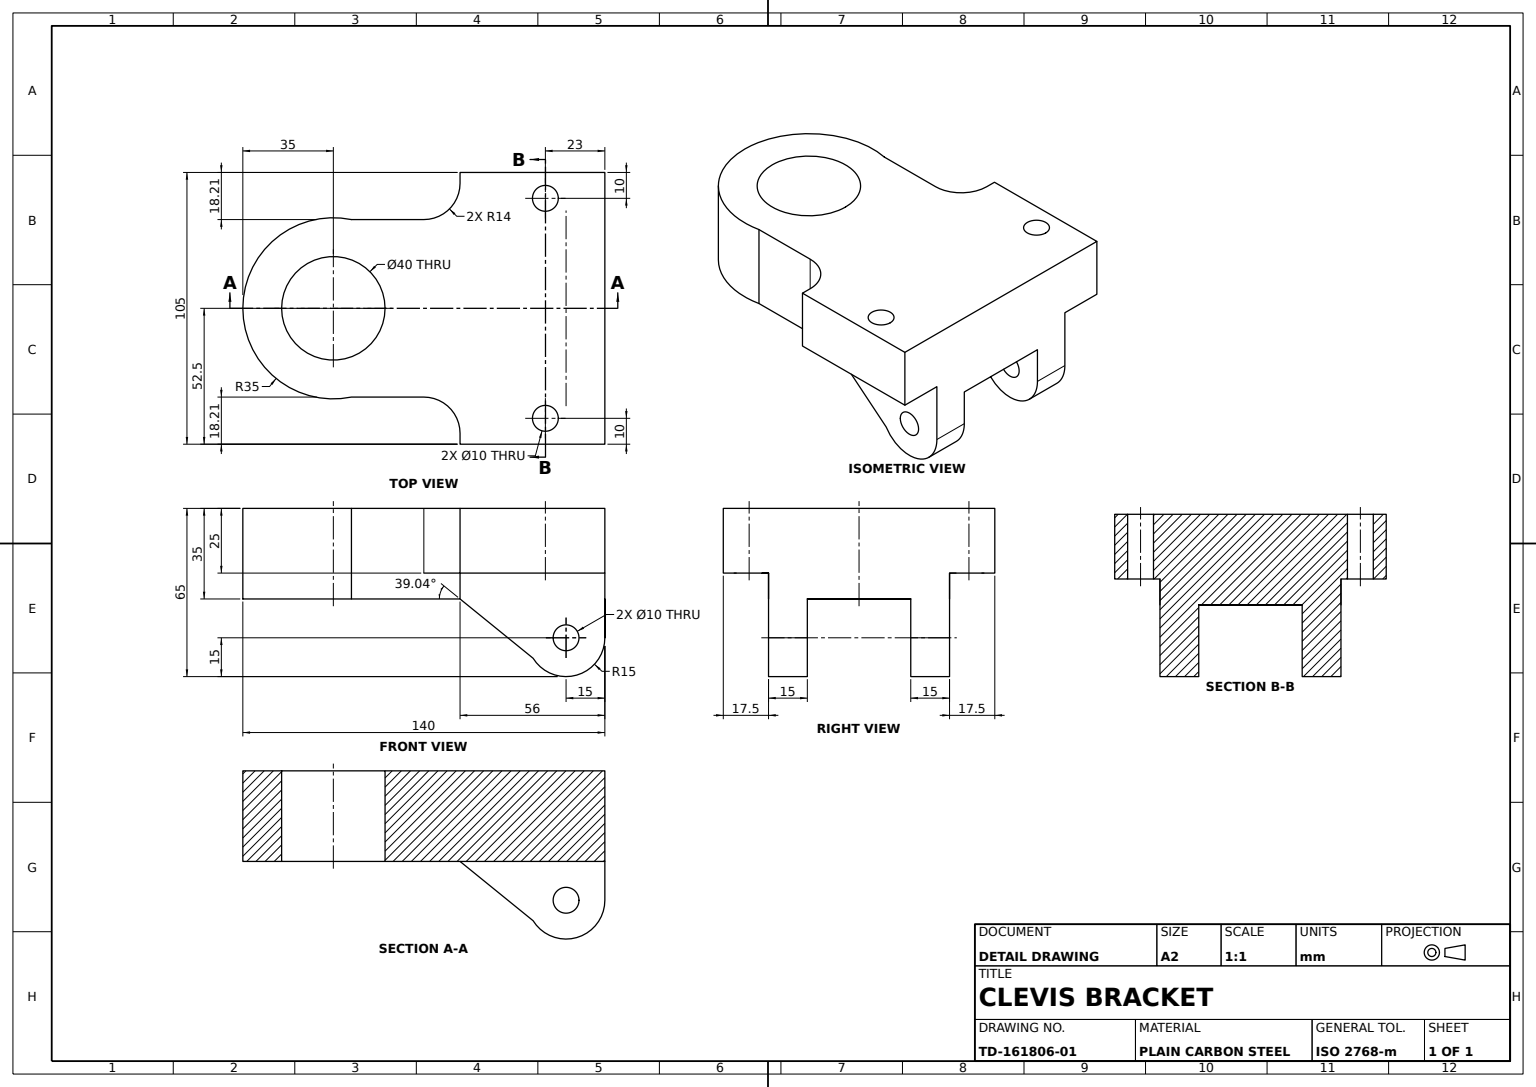
from build123d import *
from build123d.topology import SkipClean

# Parameters (mm, degrees)
BASE_PLATE_SKETCH_140X105_W  = 105
BASE_PLATE_SKETCH_140X105_H  = 140
BASE_PLATE_DEPTH             = 12.5
HUB_BOSS_DEPTH               = 35
BORE_RELIEF_56_DEPTH         = 95.240384125
FILLER_START                 = -35
FILLER_BOSS_DEPTH            = 35
LUG_BOSS_DEPTH               = 25
SIDE_START                   = 20
SIDE_EAR_SKETCH_R            = 5
SIDE_EAR_DEPTH               = 15
MOUNTING_HOLES_SKETCH_10_R   = 5
MOUNTING_HOLES_SKETCH_10_R_2 = 20
MOUNTING_HOLES_10_DEPTH      = 110.001146783


with BuildPart() as part:
    # Base Plate Sketch 140x105 → Base Plate (new, symmetric)
    with BuildSketch(Plane(origin=(0, 0, 0), x_dir=(1, 0, 0), z_dir=(0, 1, 0))):
        Rectangle(BASE_PLATE_SKETCH_140X105_W, BASE_PLATE_SKETCH_140X105_H)
    extrude(amount=BASE_PLATE_DEPTH, both=True)

    # Hub Boss Sketch → Hub Boss (add)
    with BuildSketch(Plane(origin=(0, 12.5, 0), x_dir=(1, 0, 0), z_dir=(0, 1, 0))):
        with BuildLine():
            Line((-17.5, 70), (-35, 70))
            Line((-35, 70), (-35, 14))
            Line((-35, 14), (-35, -35))
            ThreePointArc((-35, -35), (-24.748737337, -59.748737346), (1.3e-08, -70))
            ThreePointArc((1.3e-08, -70), (24.748737346, -59.748737337), (35, -35))
            Line((35, -35), (35, 14))
            Line((35, 14), (35, 70))
            Line((35, 70), (17.5, 70))
            Line((17.5, 70), (-17.5, 70))
        make_face()
    extrude(amount=-HUB_BOSS_DEPTH)

    # Bore Relief Sketch _56 → Bore Relief _56 (cut, through all)
    with SkipClean():  # the faces are left unmerged after this step: merging them gives an invalid solid
        with BuildSketch(Plane(origin=(0, 12.5, 0), x_dir=(1, 0, 0), z_dir=(0, 1, 0))):
            with BuildLine():
                Line((-52.5, -70), (6e-09, -70))
                ThreePointArc((6e-09, -70), (-24.748737339, -59.748737344), (-35, -35))
                ThreePointArc((-35, -35), (-32.267021942, -21.441264992), (-24.494897428, -10))
                ThreePointArc((-24.494897428, -10), (-21.331375002, 5.291502622), (-34.292856399, 14))
                Line((-34.292856399, 14), (-52.5, 14))
                Line((-52.5, 14), (-52.5, -70))
            make_face()
            with BuildLine():
                Line((52.5, -70), (52.5, 14))
                Line((52.5, 14), (34.292856399, 14))
                ThreePointArc((34.292856399, 14), (21.331375002, 5.291502622), (24.494897428, -10))
                ThreePointArc((24.494897428, -10), (32.267021942, -21.441264992), (35, -35))
                ThreePointArc((35, -35), (24.748737344, -59.748737339), (6e-09, -70))
                Line((6e-09, -70), (52.5, -70))
            make_face()
        extrude(amount=-BORE_RELIEF_56_DEPTH, mode=Mode.SUBTRACT)

    # Filler Boss Sketch → Filler Boss (add)
    with SkipClean():  # the faces are left unmerged after this step: merging them gives an invalid solid
        with BuildSketch(Plane.XZ.offset(22.5).offset(FILLER_START)):
            with BuildLine():
                Line((-34.292856399, -14), (-34.292856399, 28))
                ThreePointArc((-34.292856399, 28), (-30.740852298, 18.266799469), (-24.494897428, 10))
                ThreePointArc((-24.494897428, 10), (-21.331375002, -5.291502622), (-34.292856399, -14))
            make_face()
            with BuildLine():
                Line((34.292856399, -14), (34.292856399, 28))
                ThreePointArc((34.292856399, 28), (30.740852298, 18.266799469), (24.494897428, 10))
                ThreePointArc((24.494897428, 10), (21.331375002, -5.291502622), (34.292856399, -14))
            make_face()
        extrude(amount=FILLER_BOSS_DEPTH)

    # Lug Boss Sketch → Lug Boss (add)
    with SkipClean():  # the faces are left unmerged after this step: merging them gives an invalid solid
        with BuildSketch(Plane(origin=(0, 12.5, 0), x_dir=(1, 0, 0), z_dir=(0, 1, 0))):
            with BuildLine():
                Line((48.292856399, 14), (34.292856399, 14))
                Line((34.292856399, 14), (34.292856399, 0))
                ThreePointArc((34.292856399, 0), (38.393361462, 9.899494937), (48.292856399, 14))
            make_face()
            with BuildLine():
                Line((-34.292856399, 0), (-34.292856399, 14))
                Line((-34.292856399, 14), (-48.292856399, 14))
                ThreePointArc((-48.292856399, 14), (-38.393361462, 9.899494937), (-34.292856399, 0))
            make_face()
        extrude(amount=-LUG_BOSS_DEPTH)

    # Side Ear Sketch → Side Ear (add)
    with SkipClean():  # the faces are left unmerged after this step: merging them gives an invalid solid
        with BuildSketch(Plane(origin=(0, 0, 0), x_dir=(0, 0, -1), z_dir=(1, 0, 0)).offset(SIDE_START)):
            with BuildLine():
                Line((70, -37.5), (70, -22.5))
                Line((70, -22.5), (14, -22.5))
                Line((14, -22.5), (42.254134702, -45.408408045))
                ThreePointArc((42.254134702, -45.408408045), (47.707062344, -50.607748103), (55, -52.5))
                ThreePointArc((55, -52.5), (65.606601718, -48.106601718), (70, -37.5))
            make_face()
            with Locations((55, -37.5)):
                Circle(SIDE_EAR_SKETCH_R, mode=Mode.SUBTRACT)
        side_ear = extrude(amount=SIDE_EAR_DEPTH)

    # Side Ear Mirror: Side Ear across plane
    with SkipClean():  # the faces are left unmerged after this step: merging them gives an invalid solid
        add(side_ear.mirror(Plane(origin=(0, 0, 0), x_dir=(0, 0, 1), z_dir=(1, 0, 0))))

    # Mounting Holes Sketch _10 → Mounting Holes _10 (cut, through all)
    with SkipClean():  # the faces are left unmerged after this step: merging them gives an invalid solid
        with BuildSketch(Plane(origin=(0, 12.5, 0), x_dir=(1, 0, 0), z_dir=(0, 1, 0))):
            with Locations(Location((-42.5, 47, 0), (0, 0, 270))):
                Circle(MOUNTING_HOLES_SKETCH_10_R)
            with Locations(Location((42.5, 47, 0), (0, 0, 270))):
                Circle(MOUNTING_HOLES_SKETCH_10_R)
            with Locations(Location((0, -35, 0), (0, 0, 270))):
                Circle(MOUNTING_HOLES_SKETCH_10_R_2)
        extrude(amount=-MOUNTING_HOLES_10_DEPTH, mode=Mode.SUBTRACT)


solid = part.part
